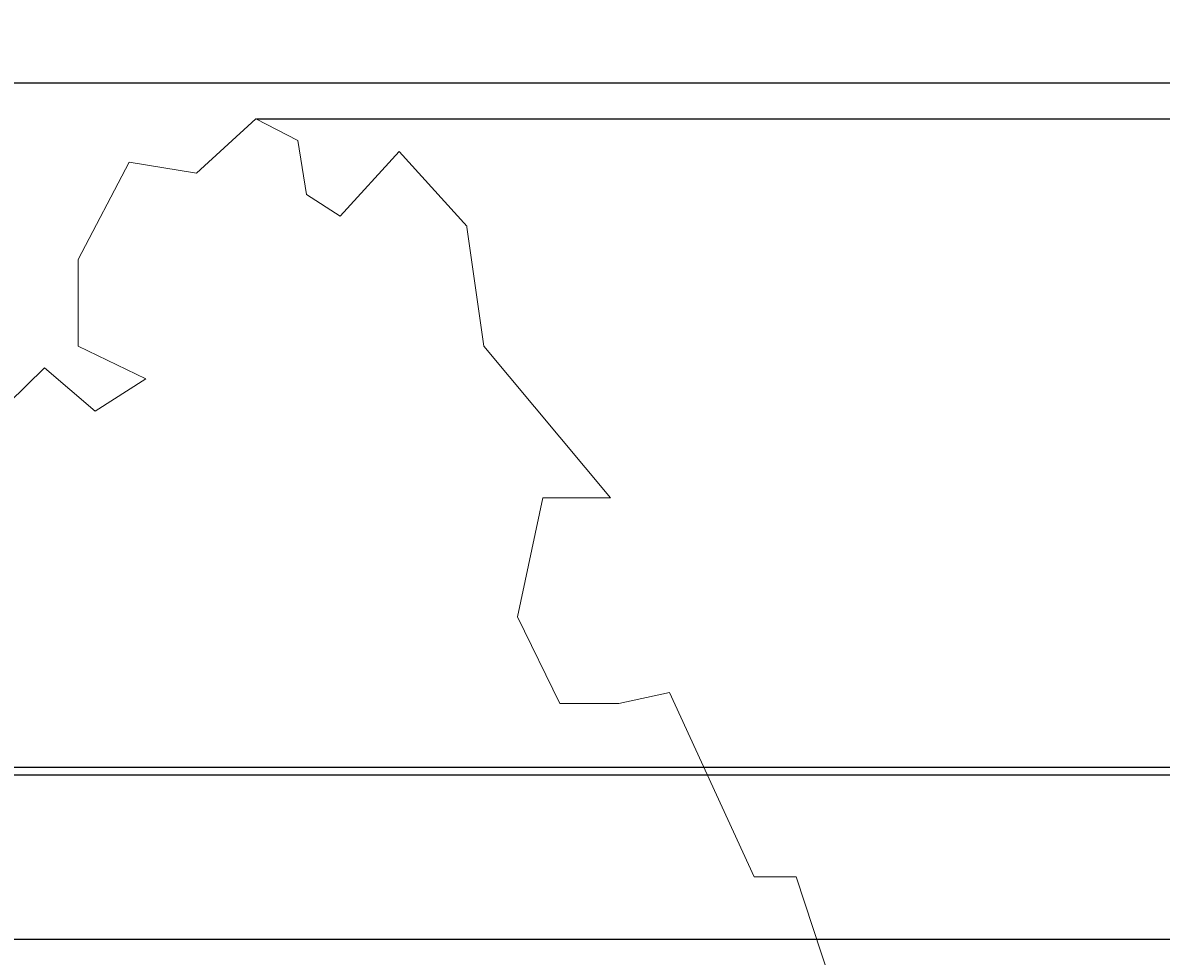
# Model space of a CAD drawing. Units: inches. Extents: x -26 to 776, y -22 to 650.
# Tile 54 of 62: x 642 to 724, y 158 to 226. Entities that reach past the tile are written whole.
import ezdxf

# ---------------------------------------------------------------- set-up
doc = ezdxf.new("R2010")
doc.units = ezdxf.units.IN
doc.header["$MEASUREMENT"] = 0
doc.layers.add('A-ANNO-DIMS', color=2, linetype='Continuous', lineweight=18)
doc.layers.add('L-PLNT-TREE', color=94, linetype='Continuous', lineweight=18)
doc.styles.get("Standard").update_dxf_attribs({"font": 'arial.ttf'})
doc.dimstyles.get("Standard").update_dxf_attribs({"dimtxt": 0.5625, "dimasz": 0.18, "dimexe": 0.18, "dimexo": 0.0625, "dimgap": 0.09, "dimtad": 0, "dimtih": 1, "dimtoh": 1, "dimdec": 4, "dimzin": 0, "dimdsep": 46, "dimlunit": 4, "dimtxsty": 'Standard', "dimcen": 0.09, "dimadec": 0, "dimazin": 0, "dimtfac": 1, "dimtdec": 4, "dimtofl": 0, "dimtmove": 0, "dimatfit": 3, "dimfxl": 1, "dimtolj": 1, "dimtzin": 0, "dimarcsym": 0})

# ---------------------------------------------------------------- blocks, each defined once
blk = doc.blocks.new('Tree - type 3 evergreen elevation')
for points in [[(22.0124, 137.721), (18.5475, 141.5624), (15.5282, 138.2446), (13.8028, 139.3505), (13.3714, 142.1153), (11.2148, 143.2214), (8.1954, 140.4564), (4.7447, 141.0094), (2.1567, 136.0326), (2.1567, 131.6088), (5.6074, 129.9499), (3.0193, 128.2909), (0.4313, 130.5029), (-6.9015, 123.3141)], [(42.2711, 94.0063), (38.8204, 104.5129), (36.6637, 104.5129), (32.3503, 113.9135), (29.7623, 113.3605), (26.743, 113.3605), (24.5862, 117.7844), (25.8802, 123.8671), (29.331, 123.8671), (22.8609, 131.6088), (21.9982, 137.6916)]]:
    blk.add_lwpolyline(points)
blk = doc.blocks.new('*D20')
at = {"layer": 'A-ANNO-DIMS', "color": 0, "lineweight": -2, "transparency": 16777216}
for p, q in [((425.806, 455.472), (775.335, 455.472)), ((775.155, 455.292), (775.155, 235.854)), ((775.155, 15.662), (775.155, 235.1)), ((425.806, 15.482), (775.335, 15.482))]:
    blk.add_line(p, q, dxfattribs=at)
at = {"layer": 'A-ANNO-DIMS', "color": 0, "transparency": 16777216}
for points in [[(775.125, 455.292), (775.185, 455.292), (775.155, 455.472)], [(775.125, 15.662), (775.185, 15.662), (775.155, 15.482)]]:
    blk.add_solid(points, dxfattribs=at)
at = {"layer": 'Defpoints', "color": 0, "transparency": 16777216}
for p in [(425.743, 455.472), (775.155, 455.472), (425.743, 15.482)]:
    blk.add_point(p, dxfattribs=at)
at = {"layer": 'A-ANNO-DIMS', "color": 0, "transparency": 16777216, "insert": (775.155, 235.477), "char_height": 0.5625, "attachment_point": 5}
blk.add_mtext('\\A1;440', dxfattribs=at)
blk = doc.blocks.new('*D26')
at = {"layer": 'A-ANNO-DIMS', "color": 0, "lineweight": -2, "transparency": 16777216}
for p, q in [((91.707, 171.973), (775.335, 171.973)), ((775.155, 171.793), (775.155, 166.105)), ((775.155, 159.662), (775.155, 165.351)), ((82.196, 159.482), (775.335, 159.482))]:
    blk.add_line(p, q, dxfattribs=at)
at = {"layer": 'A-ANNO-DIMS', "color": 0, "transparency": 16777216}
for points in [[(775.125, 171.793), (775.185, 171.793), (775.155, 171.973)], [(775.125, 159.662), (775.185, 159.662), (775.155, 159.482)]]:
    blk.add_solid(points, dxfattribs=at)
at = {"layer": 'Defpoints', "color": 0, "transparency": 16777216}
for p in [(91.645, 171.973), (775.155, 171.973), (82.134, 159.482)]:
    blk.add_point(p, dxfattribs=at)
at = {"layer": 'A-ANNO-DIMS', "color": 0, "transparency": 16777216, "insert": (775.155, 165.728), "char_height": 0.5625, "attachment_point": 5}
blk.add_mtext('\\A1;12.49', dxfattribs=at)
blk = doc.blocks.new('*D28')
at = {"layer": 'A-ANNO-DIMS', "color": 0, "lineweight": -2, "transparency": 16777216}
for p, q in [((285.08, 314.119), (775.335, 314.119)), ((775.155, 313.939), (775.155, 243.141)), ((775.155, 171.597), (775.155, 242.396)), ((285.08, 171.417), (775.335, 171.417))]:
    blk.add_line(p, q, dxfattribs=at)
at = {"layer": 'A-ANNO-DIMS', "color": 0, "transparency": 16777216}
for points in [[(775.125, 313.939), (775.185, 313.939), (775.155, 314.119)], [(775.125, 171.597), (775.185, 171.597), (775.155, 171.417)]]:
    blk.add_solid(points, dxfattribs=at)
at = {"layer": 'Defpoints', "color": 0, "transparency": 16777216}
for p in [(285.018, 314.119), (775.155, 314.119), (285.018, 171.417)]:
    blk.add_point(p, dxfattribs=at)
at = {"layer": 'A-ANNO-DIMS', "color": 0, "transparency": 16777216, "insert": (775.155, 242.768), "char_height": 0.5625, "attachment_point": 5}
blk.add_mtext('\\A1;142.7', dxfattribs=at)
blk = doc.blocks.new('*D41')
at = {"layer": 'A-ANNO-DIMS', "color": 0, "lineweight": -2, "transparency": 16777216}
for p, q in [((11.17, 221.641), (775.335, 221.641)), ((775.155, 221.461), (775.155, 190.939)), ((775.155, 159.662), (775.155, 190.185)), ((11.17, 159.482), (775.335, 159.482))]:
    blk.add_line(p, q, dxfattribs=at)
at = {"layer": 'A-ANNO-DIMS', "color": 0, "transparency": 16777216}
for points in [[(775.125, 221.461), (775.185, 221.461), (775.155, 221.641)], [(775.125, 159.662), (775.185, 159.662), (775.155, 159.482)]]:
    blk.add_solid(points, dxfattribs=at)
at = {"layer": 'Defpoints', "color": 0, "transparency": 16777216}
for p in [(11.107, 221.641), (775.155, 221.641), (11.107, 159.482)]:
    blk.add_point(p, dxfattribs=at)
at = {"layer": 'A-ANNO-DIMS', "color": 0, "transparency": 16777216, "insert": (775.155, 190.562), "char_height": 0.5625, "attachment_point": 5}
blk.add_mtext('\\A1;62.16', dxfattribs=at)
blk = doc.blocks.new('*D42')
at = {"layer": 'A-ANNO-DIMS', "color": 0, "lineweight": -2, "transparency": 16777216}
for p, q in [((285.08, 171.417), (775.335, 171.417)), ((775.155, 171.237), (775.155, 165.827)), ((775.155, 159.662), (775.155, 165.072)), ((289.305, 159.482), (775.335, 159.482))]:
    blk.add_line(p, q, dxfattribs=at)
at = {"layer": 'A-ANNO-DIMS', "color": 0, "transparency": 16777216}
for points in [[(775.125, 171.237), (775.185, 171.237), (775.155, 171.417)], [(775.125, 159.662), (775.185, 159.662), (775.155, 159.482)]]:
    blk.add_solid(points, dxfattribs=at)
at = {"layer": 'Defpoints', "color": 0, "transparency": 16777216}
for p in [(285.018, 171.417), (775.155, 171.417), (289.242, 159.482)]:
    blk.add_point(p, dxfattribs=at)
at = {"layer": 'A-ANNO-DIMS', "color": 0, "transparency": 16777216, "insert": (775.155, 165.45), "char_height": 0.5625, "attachment_point": 5}
blk.add_mtext('\\A1;11.935', dxfattribs=at)
blk = doc.blocks.new('*D45')
at = {"layer": 'A-ANNO-DIMS', "color": 0, "lineweight": -2, "transparency": 16777216}
for p, q in [((507.738, 408.639), (775.335, 408.639)), ((775.155, 408.459), (775.155, 212.438)), ((775.155, 15.662), (775.155, 211.683)), ((585.998, 15.482), (775.335, 15.482))]:
    blk.add_line(p, q, dxfattribs=at)
at = {"layer": 'A-ANNO-DIMS', "color": 0, "transparency": 16777216}
for points in [[(775.125, 408.459), (775.185, 408.459), (775.155, 408.639)], [(775.125, 15.662), (775.185, 15.662), (775.155, 15.482)]]:
    blk.add_solid(points, dxfattribs=at)
at = {"layer": 'Defpoints', "color": 0, "transparency": 16777216}
for p in [(507.676, 408.639), (775.155, 408.639), (585.935, 15.482)]:
    blk.add_point(p, dxfattribs=at)
at = {"layer": 'A-ANNO-DIMS', "color": 0, "transparency": 16777216, "insert": (775.155, 212.061), "char_height": 0.5625, "attachment_point": 5}
blk.add_mtext('\\A1;393.16', dxfattribs=at)
blk = doc.blocks.new('*D46')
at = {"layer": 'A-ANNO-DIMS', "color": 0, "lineweight": -2, "transparency": 16777216}
for p, q in [((658.506, 219.032), (775.335, 219.032)), ((775.155, 218.852), (775.155, 117.635)), ((775.155, 15.662), (775.155, 116.88)), ((677.966, 15.482), (775.335, 15.482))]:
    blk.add_line(p, q, dxfattribs=at)
at = {"layer": 'A-ANNO-DIMS', "color": 0, "transparency": 16777216}
for points in [[(775.125, 218.852), (775.185, 218.852), (775.155, 219.032)], [(775.125, 15.662), (775.185, 15.662), (775.155, 15.482)]]:
    blk.add_solid(points, dxfattribs=at)
at = {"layer": 'Defpoints', "color": 0, "transparency": 16777216}
for p in [(658.444, 219.032), (775.155, 219.032), (677.904, 15.482)]:
    blk.add_point(p, dxfattribs=at)
at = {"layer": 'A-ANNO-DIMS', "color": 0, "transparency": 16777216, "insert": (775.155, 117.257), "char_height": 0.5625, "attachment_point": 5}
blk.add_mtext('\\A1;203.55', dxfattribs=at)
blk = doc.blocks.new('*D48')
at = {"layer": 'A-ANNO-DIMS', "color": 0, "lineweight": -2, "transparency": 16777216}
for p, q in [((545.033, 67.415), (545.033, 649.856)), ((545.213, 649.676), (640.879, 649.676)), ((738.57, 649.676), (642.904, 649.676)), ((738.75, 50.911), (738.75, 649.856))]:
    blk.add_line(p, q, dxfattribs=at)
at = {"layer": 'A-ANNO-DIMS', "color": 0, "transparency": 16777216}
for points in [[(545.213, 649.706), (545.213, 649.646), (545.033, 649.676)], [(738.57, 649.706), (738.57, 649.646), (738.75, 649.676)]]:
    blk.add_solid(points, dxfattribs=at)
at = {"layer": 'Defpoints', "color": 0, "transparency": 16777216}
for p in [(738.75, 649.676), (545.033, 67.352), (738.75, 50.848)]:
    blk.add_point(p, dxfattribs=at)
at = {"layer": 'A-ANNO-DIMS', "color": 0, "transparency": 16777216, "insert": (641.892, 649.676), "char_height": 0.5625, "attachment_point": 5}
blk.add_mtext('\\A1;193.7', dxfattribs=at)

msp = doc.modelspace()

# ---------------------------------------------------------------- block references
at = {"layer": 'L-PLNT-TREE', "xscale": 1.421226385586178, "yscale": 1.421226385586178, "zscale": 1.421226385586178}
msp.add_blockref('Tree - type 3 evergreen elevation', (642.5048, 15.4824), dxfattribs=at)

# ---------------------------------------------------------------- dimensions: what is measured, and where the dimension line sits
at = {"layer": 'A-ANNO-DIMS'}
dim = msp.add_linear_dim(base=(738.7503, 649.6763), p1=(545.0331, 67.3523), p2=(738.7503, 50.8482), dimstyle='Standard', override={"dimdec": 1, "dimlfac": 1, "dimrnd": 0, "dimzin": 0, "dimdsep": 46, "dimlunit": 2}, dxfattribs=at)
dim.commit()
dim.dimension.update_dxf_attribs({"geometry": '*D48', "text_midpoint": (641.8917, 649.6763)})
for base, p1, p2, override, picture, middle in [((775.1553, 455.4717), (425.7434, 15.4824), (425.7434, 455.4717), {"dimdec": 0, "dimlfac": 1, "dimrnd": 0, "dimzin": 0, "dimdsep": 46, "dimlunit": 2}, '*D20', (775.1553, 235.477)), ((775.1553, 408.6389), (585.9354, 15.4824), (507.6759, 408.6389), {"dimdec": 2, "dimlfac": 1, "dimrnd": 0, "dimzin": 0, "dimdsep": 46, "dimlunit": 2}, '*D45', (775.1553, 212.0606)), ((775.1553, 314.119), (285.0179, 171.4173), (285.0179, 314.119), {"dimdec": 1, "dimlfac": 1, "dimrnd": 0, "dimzin": 0, "dimdsep": 46, "dimlunit": 2}, '*D28', (775.1553, 242.7682)), ((775.1553, 221.6413), (11.1074, 159.4824), (11.1074, 221.6413), {"dimdec": 2, "dimlfac": 1, "dimrnd": 0, "dimzin": 0, "dimdsep": 46, "dimlunit": 2}, '*D41', (775.1553, 190.5618)), ((775.1553, 219.0324), (677.9037, 15.4824), (658.4435, 219.0324), {"dimdec": 2, "dimlfac": 1, "dimrnd": 0, "dimzin": 0, "dimdsep": 46, "dimlunit": 2}, '*D46', (775.1553, 117.2574)), ((775.1553, 171.9734), (82.134, 159.4824), (91.6448, 171.9734), {"dimdec": 2, "dimlfac": 1, "dimrnd": 0, "dimzin": 0, "dimdsep": 46, "dimlunit": 2}, '*D26', (775.1553, 165.7279)), ((775.1553, 171.4173), (289.2424, 159.4824), (285.0179, 171.4173), {"dimdec": 3, "dimlfac": 1, "dimrnd": 0, "dimzin": 0, "dimdsep": 46, "dimlunit": 2}, '*D42', (775.1553, 165.4498))]:
    dim = msp.add_linear_dim(base=base, p1=p1, p2=p2, angle=90, dimstyle='Standard', override=override, dxfattribs=at)
    dim.commit()
    dim.dimension.update_dxf_attribs({"geometry": picture, "text_midpoint": middle})

doc.saveas('drawing.dxf')
